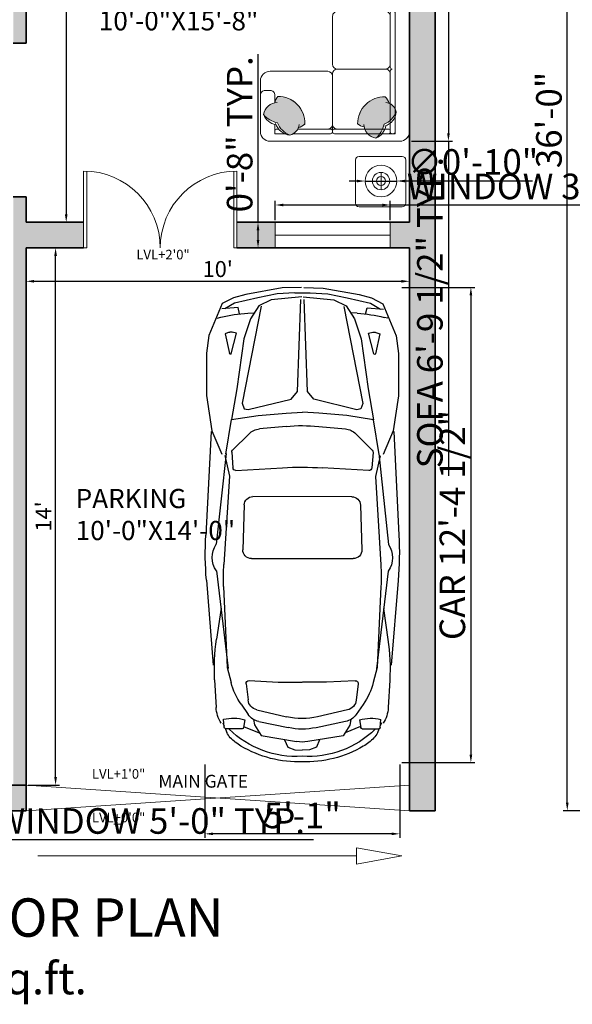
# Model space of a CAD drawing. Units: inches. Extents: x 3259 to 4981, y 1402 to 2026.
# Tile 2 of 11: x 3471 to 3644, y 1415 to 1722. Entities that reach past the tile are written whole.
import ezdxf

# ---------------------------------------------------------------- set-up
doc = ezdxf.new("R2010")
doc.units = ezdxf.units.IN
for name, color, linetype, lineweight in [('A-ANNO-DIMS', 2, 'Continuous', 13), ('A-ANNO-SYMB', 7, 'Continuous', 13), ('A-ANNO-TEXT', 7, 'Continuous', 18), ('A-ANNO-TITL', 7, 'Continuous', 25), ('A-AREA-IDEN', 7, 'Continuous', 18), ('A-DOOR', 3, 'Continuous', 18), ('A-FURN', 8, 'Continuous', 13), ('A-GLAZ', 4, 'Continuous', 18), ('A-VEHI', 8, 'Continuous', 13), ('A-WALL', 7, 'Continuous', 35), ('A-WALL-PATT', 252, 'Continuous', 13)]:
    doc.layers.add(name, color=color, linetype=linetype, lineweight=lineweight)
doc.layers.add('L9012X$0', color=2, linetype='Continuous')
doc.styles.get("Standard").update_dxf_attribs({"font": 'arial.ttf'})
doc.dimstyles.new('ISO-25', dxfattribs={"dimtxt": 8, "dimasz": 2.5, "dimexe": 1.25, "dimexo": 0.625, "dimtad": 1, "dimdec": 1, "dimlunit": 3, "dimtxsty": 'Standard', "dimcen": 2.5, "dimclrd": 4, "dimclre": 4, "dimclrt": 1, "dimadec": 0, "dimazin": 0, "dimtfac": 1, "dimtdec": 1, "dimtmove": 0, "dimatfit": 3, "dimfxl": 1, "dimarcsym": 0})

# ---------------------------------------------------------------- blocks, each defined once
blk = doc.blocks.new('SOFA 1')
at = {"transparency": 33554687}
h = blk.add_hatch(color=256, dxfattribs=at)
h.dxf.hatch_style = 1
h.paths.add_polyline_path([(3723.52, 1308.63, 0.147724), (3717.76, 1305.24, 0.310469), (3722.42, 1300.4), (3722.42, 1300.25, 0.156703), (3723.62, 1297.8, 0.425821), (3734.69, 1309.08, 0.121928), (3732.05, 1310.63, 0.233216), (3728.6, 1313.59, 0.213835)])
h = blk.add_hatch(color=256, dxfattribs=at)
h.dxf.hatch_style = 1
h.paths.add_polyline_path([(3769.65, 1307.6, 0.084911), (3767.15, 1309.12, 0.046133), (3766.46, 1311.13), (3759.18, 1311.13, 0.039409), (3758.92, 1310.24, 0.165523), (3756.31, 1309.02, 0.42585), (3767.59, 1297.95, 0.121928), (3769.15, 1300.58, 0.027403), (3769.65, 1300.83)])
h.paths.add_polyline_path([(3765.34, 1313.08), (3760.4, 1313.08, 0.097704), (3759.18, 1311.13), (3766.46, 1311.13, 0.04873)])
h.paths.add_polyline_path([(3763.76, 1314.88, 0.16488), (3760.4, 1313.08), (3765.34, 1313.08, 0.051917)])
h.paths.add_polyline_path([(3771.6, 1305.17, 0.090388), (3769.65, 1307.6), (3769.65, 1300.83, 0.136035), (3771.6, 1302.77)])
h = blk.add_hatch(color=256, dxfattribs=at)
h.dxf.hatch_style = 1
h.paths.add_polyline_path([(3769.16, 1235.96, 0.122267), (3767.6, 1238.61, 0.425972), (3756.32, 1227.54, 0.165563), (3758.93, 1226.32, 0.309481), (3763.76, 1221.69, 0.002677), (3763.83, 1221.72, 0.146094), (3767.16, 1227.43, 0.212433), (3772.1, 1232.48, 0.235342)])
h = blk.add_hatch(color=256, dxfattribs=at)
h.dxf.hatch_style = 1
h.paths.add_polyline_path([(3769.16, 1225.36, 0.122267), (3767.6, 1228.01, 0.425972), (3756.32, 1216.94, 0.165563), (3758.93, 1215.72, 0.309481), (3763.76, 1211.09, 0.002677), (3763.83, 1211.12, 0.146094), (3767.16, 1216.83, 0.212433), (3772.1, 1221.88, 0.235342)])
for p, q in [((3720.45, 1316.13), (3773.58, 1316.13)), ((3777.51, 1312.19), (3777.51, 1213.72))]:
    blk.add_line(p, q, dxfattribs=at)
for points in [[(3717.76, 1305.24, -0.147724), (3723.52, 1308.63, -0.213355), (3728.59, 1313.59, 0.213355), (3723.52, 1308.63, 0.147724), (3717.76, 1305.24, -0.249545), (3722.86, 1309.34, 0.249545), (3717.75, 1305.25, 0.356779), (3723.4, 1300.28, -0.356779), (3717.76, 1305.24)], [(3728.58, 1313.6, -0.306333), (3732.42, 1309.31, 0.306333), (3728.58, 1313.6, 0.306674), (3722.72, 1308.89, -0.306674), (3728.58, 1313.6)], [(3763.76, 1314.88, -0.147724), (3767.15, 1309.12, -0.213355), (3772.1, 1304.05, 0.213355), (3767.15, 1309.12, 0.147724), (3763.76, 1314.88, -0.249545), (3767.86, 1309.77, 0.249545), (3763.77, 1314.89, 0.356779), (3758.8, 1309.23, -0.356779), (3763.76, 1314.88)], [(3734.69, 1309.08, -0.425972), (3723.62, 1297.8, -0.165552), (3722.4, 1300.4, 0.165552), (3723.62, 1297.79, 0.425972), (3734.69, 1309.07, 0.121514), (3732.07, 1310.63, -0.121514), (3734.69, 1309.08)], [(3767.6, 1297.95, -0.425972), (3756.31, 1309.01, -0.165552), (3758.92, 1310.24, 0.165552), (3756.31, 1309.02, 0.425972), (3767.59, 1297.95, 0.121514), (3769.14, 1300.57, -0.121514), (3767.6, 1297.95)], [(3772.11, 1304.06, -0.306333), (3767.83, 1300.22, 0.306333), (3772.11, 1304.06, 0.306674), (3767.4, 1309.91, -0.306674), (3772.11, 1304.06)], [(3770.44, 1286.63, -0.414214), (3769.66, 1287.4, 0.414214), (3770.44, 1286.63, 0.414214), (3769.66, 1285.83, -0.414214), (3770.44, 1286.63)], [(3748.01, 1262.99, -0.414214), (3746.05, 1264.95, 0.414214), (3748.01, 1262.97, 0.414213), (3746.05, 1261.01, -0.414213), (3748.01, 1262.99)], [(3770.44, 1262.99, -0.414214), (3769.66, 1263.77, 0.414214), (3770.44, 1262.99, 0.414214), (3769.66, 1262.19, -0.414214), (3770.44, 1262.99)], [(3770.83, 1262.97, -0.414214), (3771.61, 1262.19, 0.414214), (3770.83, 1262.99, 0.414214), (3771.61, 1263.77, -0.414214), (3770.83, 1262.97)], [(3748.01, 1239.35, -0.414214), (3746.05, 1241.31, 0.414214), (3748.01, 1239.33, 0.414213), (3746.05, 1237.37, -0.414213), (3748.01, 1239.35)], [(3767.7, 1239.33, -0.414214), (3769.66, 1237.37, 0.414214), (3767.7, 1239.35, 0.414214), (3769.66, 1241.31, -0.414214), (3767.7, 1239.33)], [(3756.32, 1227.54, -0.425972), (3767.6, 1238.61, -0.121514), (3769.16, 1235.98, 0.121514), (3767.6, 1238.61, 0.425972), (3756.32, 1227.54, 0.165552), (3758.93, 1226.32, -0.165552), (3756.32, 1227.54)], [(3770.44, 1239.35, -0.414214), (3769.66, 1240.13, 0.414214), (3770.44, 1239.33, 0.414214), (3769.66, 1238.55, -0.414214), (3770.44, 1239.35)], [(3770.83, 1239.33, -0.414214), (3771.61, 1238.55, 0.414214), (3770.83, 1239.35, 0.414214), (3771.61, 1240.13, -0.414214), (3770.83, 1239.33)], [(3763.78, 1221.67, 0.249545), (3767.87, 1226.78, -0.249545), (3763.76, 1221.69, -0.356779), (3758.81, 1227.32, 0.356779), (3763.77, 1221.68, 0.147724), (3767.16, 1227.43, 0.213355), (3772.11, 1232.51, -0.213355), (3767.16, 1227.43, -0.147724), (3763.78, 1221.67)], [(3772.1, 1232.5, -0.306674), (3767.41, 1226.64, 0.306674), (3772.1, 1232.5, 0.306333), (3767.84, 1236.34, -0.306333), (3772.1, 1232.5)], [(3756.32, 1216.94, -0.200233), (3759.49, 1224.76, 0.200233), (3756.32, 1216.94, 0.165552), (3758.93, 1215.72, -0.165552), (3756.32, 1216.94)], [(3772.1, 1221.9, -0.306674), (3767.41, 1216.04, 0.306674), (3772.1, 1221.9, -0.213355), (3767.16, 1216.83, -0.147724), (3763.77, 1211.08, 0.147724), (3767.15, 1216.83, 0.213355), (3772.1, 1221.9)], [(3763.76, 1211.09, -0.356779), (3758.81, 1216.72, 0.356779), (3763.76, 1211.09, 0.249545), (3767.87, 1216.18, -0.249545), (3763.76, 1211.09)]]:
    blk.add_lwpolyline(points, format="xyb", dxfattribs=at)
for points in [[(3722.42, 1313.08), (3722.42, 1309.23), (3722.42, 1313.08), (3726.57, 1313.08)], [(3729.85, 1313.08), (3745.25, 1313.08)], [(3768.11, 1313.08), (3746.78, 1313.08)], [(3771.6, 1313.08), (3767.75, 1313.08), (3771.6, 1313.08), (3771.6, 1308.93)], [(3771.6, 1313.08), (3771.61, 1233.74)], [(3716.51, 1312.2), (3716.51, 1291.44)], [(3723.21, 1311.13), (3723.93, 1311.13)], [(3731.82, 1311.13), (3745.25, 1311.13)], [(3746.01, 1312.3), (3746.01, 1288.55)], [(3746.01, 1310.97), (3746.01, 1311.36)], [(3768.87, 1311.13), (3746.78, 1311.13)], [(3769.66, 1287.39), (3769.65, 1312.3)], [(3769.65, 1309.43), (3769.65, 1308.71)], [(3746.01, 1288.54), (3746.01, 1308.23)], [(3722.42, 1300.39), (3722.42, 1297.33)], [(3720.45, 1295.38), (3718.48, 1295.38)], [(3720.45, 1287.5), (3744.09, 1287.5)], [(3747.99, 1286.6), (3767.69, 1286.6)], [(3769.66, 1263.75), (3769.66, 1285.81)], [(3746.02, 1284.63), (3746.02, 1264.94)], [(3769.66, 1277.18), (3769.66, 1263.75)], [(3746.02, 1260.99), (3746.02, 1241.3)], [(3747.99, 1262.97), (3767.69, 1262.97)], [(3769.66, 1240.12), (3769.66, 1262.18)], [(3770.43, 1262.97), (3770.82, 1262.97)], [(3746.02, 1237.36), (3746.02, 1213.74)], [(3747.99, 1239.33), (3767.69, 1239.33)], [(3769.66, 1235.71), (3769.66, 1238.54)], [(3770.43, 1239.33), (3770.82, 1239.33)], [(3771.61, 1223.14), (3771.61, 1230.47)], [(3769.66, 1225.11), (3769.66, 1227.82)], [(3767.76, 1215.72), (3771.61, 1215.72), (3771.61, 1219.84), (3771.61, 1215.72)], [(3769.66, 1216.5), (3769.66, 1217.22)], [(3753.91, 1211.77), (3753.91, 1213.74)], [(3755.86, 1215.72), (3758.92, 1215.72)], [(3749.97, 1209.8), (3773.58, 1209.8)]]:
    blk.add_lwpolyline(points, close=True, dxfattribs=at)
for points in [[(3770.43, 1313.08, 0.414214), (3769.65, 1312.3, -0.414214)], [(3771.6, 1312.3, 0.414214), (3770.82, 1313.08, -0.414214)], [(3722.42, 1311.91, 0.414214), (3723.2, 1311.13, -0.414214)], [(3716.51, 1297.34, 0.414214), (3718.47, 1295.38, -0.414214)], [(3720.44, 1295.38, 0.414214), (3722.4, 1297.34, -0.414214)], [(3716.51, 1291.45, 0.414212), (3720.44, 1287.52, -0.414212)], [(3746.03, 1288.56, 0.414214), (3747.99, 1286.6, 0.414213), (3746.03, 1284.64, -0.414213), (3747.99, 1286.6, -0.414214)], [(3769.66, 1284.64, 0.414214), (3767.7, 1286.6, 0.414214), (3769.66, 1288.56, -0.414214), (3767.7, 1286.6, -0.414214)], [(3769.66, 1261.01, 0.414214), (3767.7, 1262.97, 0.414214), (3769.66, 1264.93, -0.414214), (3767.7, 1262.97, -0.414214)], [(3772.13, 1221.9, 0.306333), (3767.84, 1225.74, -0.306333)], [(3769.16, 1225.36, 0.071861), (3768.39, 1227.01, -0.071861)], [(3769.66, 1216.52, 0.414214), (3770.44, 1215.74, -0.414214)], [(3770.83, 1215.74, 0.414214), (3771.61, 1216.52, -0.414214)], [(3746.05, 1213.76, 0.414212), (3749.98, 1209.82, -0.414212)], [(3755.87, 1215.72, 0.414214), (3753.91, 1213.76, -0.414214)], [(3755.87, 1209.8, -0.414214), (3753.91, 1211.76, 0.414214)]]:
    blk.add_lwpolyline(points, format="xyb", close=True, dxfattribs=at)
for centre, radius, start, end in [((3720.44, 1312.2), 3.93, 90.0002, 179.9998), ((3720.44, 1312.19), 3.94, 89.9158, 179.9154), ((3745.22, 1312.29), 0.789, 0.8425, 90.8425), ((3746.8, 1312.29), 0.789, 89.1575, 179.1575), ((3768.87, 1312.3), 0.777, 360, 90), ((3773.58, 1312.2), 3.93, 0.0002, 89.9998), ((3773.57, 1312.19), 3.94, 359.9158, 89.9154), ((3744.09, 1309.21), 1.92, 358.766, 90.5111), ((3745.24, 1311.91), 0.777, 270, 0), ((3745.24, 1311.91), 0.777, 270, 0), ((3746.79, 1311.91), 0.777, 180, 270), ((3746.79, 1311.91), 0.777, 180, 270), ((3747.93, 1309.21), 1.92, 89.4889, 181.234), ((3768.87, 1311.91), 0.777, 270, 0), ((3744.08, 1289.48), 1.96, 270, 360), ((3744.08, 1289.48), 1.96, 270, 360), ((3773.58, 1213.73), 3.93, 270.0002, 359.9998), ((3773.59, 1213.73), 3.93, 269.9156, 359.9152)]:
    blk.add_arc(centre, radius, start, end, dxfattribs=at)
blk = doc.blocks.new('A1099DC')
at = {"color": 0, "linetype": 'ByBlock'}
for p, q in [((1279.298465, 804.448389), (2201.430588, 851.890505)), ((2602.736326, 846.078152), (3356.693814, 785.353187)), ((179.200345, 564.515703), (190.951238, 709.631982)), ((272.228253, 749.073842), (265.114727, 718.465169)), ((1475.52921, 670.226262), (2282.402739, 758.004075)), ((2519.280414, 756.817792), (3387.476361, 653.818028)), ((2851.341839, 715.213377), (3126.60716, 755.701993)), ((3488.458929, 772.663345), (3732.658862, 759.86454)), ((3867.794139, 700.329656), (3900.059395, 686.767505)), ((139.051458, 595.027331), (190.951238, 683.213377)), ((405.405047, 577.538958), (396.874865, 615.894428)), ((398.733388, 644.315148), (411.280494, 678.748261)), ((589.014326, 626.599587), (405.405047, 577.538958)), ((411.280494, 678.748261), (588.616917, 641.417897)), ((1482.852352, 674.283145), (1175.286956, 622.180789)), ((1300.814287, 466.658131), (1445.712032, 613.104998)), ((1465.665584, 620.56924), (1602.893878, 610.287296)), ((1494.603245, 682.841284), (1678.210958, 641.166865)), ((1678.210958, 641.166865), (2462.684993, 690.847736)), ((2656.476214, 692.831247), (3376.704709, 662.004075)), ((3376.704709, 662.004075), (3510.708679, 626.736433)), ((3909.27561, 688.812956), (3837.725727, 693.401722)), ((3921.162781, 527.618662), (3921.162781, 676.138994)), ((3925.383812, 676.122818), (3955.306409, 663.545364)), ((92.537504, 388.14361), (139.051458, 595.027331)), ((236.043912, 551.980927), (179.200345, 564.515703)), ((1626.354615, 583.507504), (1602.652901, 169.222264)), ((3704.596898, 536.993674), (3795.675135, 473.385795)), ((229.117398, 477.634662), (225.714299, 427.957563)), ((1933.148906, 509.557888), (2330.980062, 522.200075)), ((2409.60024, 445.938054), (2410.49349, -460.09121)), ((3493.960271, 465.734554), (3507.923021, 209.166865)), ((3522.252709, 492.345257), (3666.066199, 475.644444)), ((3841.786866, 503.451367), (3910.58243, 515.096797)), ((3901.001848, 514.780764), (3957.150905, 375.772812)), ((57.774444, 216.608726), (92.537504, 388.14361)), ((1235.045743, 136.116317), (1257.419842, 373.755108)), ((1860.238743, -448.635916), (1859.369151, 433.397797)), ((3753.293176, 397.789551), (3815.226005, 132.124765)), ((3839.396146, 426.841284), (3888.358202, 417.538958)), ((3857.610793, 379.525702), (3912.067615, 118.157673)), ((3888.358202, 417.538958), (3983.199613, 359.957848)), ((3983.199613, 359.957848), (4035.448301, 43.94997)), ((49.168662, 58.00681), (57.774444, 216.608726)), ((3507.923021, 209.166865), (3507.64153, -4.333678)), ((4019.086894, 150.376168), (4084.69605, 122.469191)), ((4084.69605, 122.469191), (4109.177079, 60.329656)), ((4109.177079, 60.329656), (4113.094043, -5.158716)), ((49.301278, -76.507426), (58.219773, -235.092064)), ((3508.347273, -221.154823), (3507.644805, -7.65525)), ((3983.920268, -371.008369), (4035.545755, -54.898082)), ((4084.948231, -133.320044), (4109.306686, -71.132359)), ((4109.306686, -71.132359), (4113.094514, -5.636391)), ((1235.330373, -152.586046), (1258.173002, -390.180259)), ((3754.088875, -409.293325), (3815.497749, -143.506937)), ((3858.370276, -390.823819), (3912.311631, -129.348921)), ((4019.394229, -161.356334), (4084.948231, -133.320044)), ((58.219773, -235.092064), (93.320996, -406.558069)), ((1627.520644, -599.204785), (1603.002095, -184.967086)), ((3494.890446, -477.749545), (3508.347273, -221.154823)), ((93.320996, -406.558069), (140.24279, -613.349673)), ((3840.248961, -438.175225), (3889.19258, -428.776374)), ((3889.19258, -428.776374), (3983.920268, -371.008369)), ((3902.027941, -525.993061), (3957.902795, -386.874665)), ((230.077082, -495.779641), (226.576036, -446.109349)), ((1301.750547, -482.997536), (1446.936772, -629.158411)), ((1934.168526, -524.650381), (2332.023837, -536.508105)), ((3523.2353, -504.304409), (3667.01558, -487.320059)), ((3705.667171, -548.593196), (3796.61981, -484.805853)), ((3842.790735, -514.780444), (3911.609128, -526.290202)), ((237.150178, -570.112104), (180.331436, -582.758939)), ((180.331436, -582.758939), (192.368445, -727.851766)), ((406.561378, -595.336142), (398.106841, -633.708356)), ((590.267037, -644.034637), (406.561378, -595.336142)), ((3922.214148, -538.79118), (3922.506998, -687.311224)), ((140.24279, -613.349673), (192.316354, -701.433212)), ((400.0214, -662.125356), (412.636377, -696.533662)), ((412.636377, -696.533662), (589.898847, -658.853701)), ((1484.19765, -690.263206), (1176.530118, -638.767405)), ((1466.905004, -636.583294), (1604.112757, -626.030785)), ((1476.866524, -686.22077), (2283.911563, -772.40743)), ((1495.965396, -698.798158), (1679.490579, -656.761786)), ((1679.490579, -656.761786), (2464.061049, -704.895745)), ((2520.786439, -770.754078), (3388.777604, -666.042617)), ((2657.855804, -706.497136), (3378.022114, -674.249887)), ((3378.022114, -674.249887), (3511.956283, -638.718087)), ((3869.186159, -711.60707), (3901.424611, -697.981326)), ((3926.727989, -687.286725), (3956.625729, -674.650294)), ((273.723073, -767.133288), (266.549207, -736.538701)), ((2852.765183, -728.494989), (3128.109803, -768.440762)), ((3489.994314, -784.688586), (3734.168535, -771.408296)), ((3910.644841, -700.0086), (3839.104145, -704.738438)), ((1280.900818, -820.829563), (2203.124693, -866.453338)), ((2604.418191, -859.849707), (3358.254477, -797.638217))]:
    blk.add_line(p, q, dxfattribs=at)
for points in [[(-0.000783, 0.794772), (5.385043, 172.701749), (63.649891, 493.818028), (92.537504, 603.957563), (144.437284, 705.166865), (428.417214, 824.236633), (585.095796, 846.190121), (961.406447, 846.190121), (1274.27399, 797.818028), (1482.852352, 709.631982)], [(83.345007, -3.206171), (111.32237, 268.957533), (164.563706, 379.583828), (279.999271, 453.709838), (456.549665, 511.628518), (901.254996, 574.918954), (1175.286956, 622.180789), (1137.52997, 385.548359), (1118.345181, 137.317882), (1109.829198, -8.358455)], [(168.178729, 359.003083), (1030.214866, 528.397865), (1077.798844, 510.531569), (1086.170082, 475.285426), (992.832238, 91.960378), (924.218938, 35.478085), (108.447994, 6.034416)], [(0.019119, -19.392451), (5.743899, -191.288474), (64.641806, -512.289243), (93.746535, -622.371603), (145.845778, -723.478374), (430.059935, -841.987962), (586.7815, -863.632471), (963.091723, -863.198028), (1275.863278, -814.209121), (1484.26735, -725.611974)], [(83.356858, -15.227176), (111.870816, -287.335185), (165.330179, -397.856284), (280.911681, -471.754535), (457.575935, -529.324983), (902.4055, -592.045995), (1176.530118, -638.767405), (1138.306616, -402.209884), (1118.632407, -154.017717), (1109.829198, -8.358455)], [(168.904615, -377.268451), (1031.273389, -545.270714), (1078.822046, -527.310627), (1087.123771, -492.048047), (993.030273, -108.907787), (924.305735, -52.560894), (108.478017, -24.418246)]]:
    blk.add_lwpolyline(points, dxfattribs=at)
for centre, radius, start, end in [((2358.037832, -2192.08357), 3048, 85.395244, 92.945173), ((2399.99649, 588.663508), 206.166238, 54.649181, 124.776949), ((1749.553982, 373.478072), 1524, 166.916578, 176.08111), ((3392.740754, -1053.630025), 1828.8, 86.999806, 98.367602), ((3718.678317, 475.802507), 284.405862, 57.329946, 87.182375), ((446.46332, 626.922805), 50.8, 159.97873, 192.538409), ((587.047263, 633.961317), 7.62, 284.960009, 78.112462), ((1463.767788, 595.240237), 25.4, 85.715073, 135.304647), ((2578.271641, -1134.295865), 1828.8, 87.549126, 93.623712), ((3355.555414, 37.211519), 609.6, 55.070043, 75.255062), ((4191.049821, 605.937201), 363.988953, 166.096081, 196.353514), ((3908.462781, 676.138994), 12.7, 0, 86.330429), ((3320.85101, 50.338397), 847.430844, 356.245089, 44.519453), ((3896.252417, 523.051998), 152.4, 46.38363, 67.20138), ((3700.933354, 318.064082), 435.542335, 30.457681, 46.38363), ((1600.996082, 584.958293), 25.4, 356.725615, 85.715073), ((3908.462781, 527.618662), 12.7, 279.607718, 0), ((3204.184594, 25.950693), 1011.814461, 358.069446, 30.457681), ((1409.148822, 359.469565), 152.4, 135.304647, 174.62136), ((1935.569151, 433.396333), 76.2, 91.82012, 179.9989), ((2333.400307, 446.03852), 76.2, 359.924458, 91.82012), ((3519.322741, 467.114813), 25.4, 83.37601, 183.115039), ((3654.346327, 374.722669), 101.6, 13.122645, 83.37601), ((3708.414764, 348.440256), 152.4, 11.769371, 55.070043), ((2752.335538, -6.739118), 1524, 174.62136, 185.491615), ((4645.676894, -4.872483), 3048, 176.725615, 183.38736), ((3221.54491, -6.276527), 609.6, 346.99033, 13.122645), ((3315.283499, -6.18411), 609.6, 348.343604, 11.769371), ((1266.577845, -8.050136), 1219.2, 176.894161, 183.218814), ((3734.73098, -5.770579), 304.8, 350.724636, 9.388339), ((3320.962449, -62.69553), 847.430844, 315.593523, 3.867886), ((3204.248172, -38.537915), 1011.814461, 329.655294, 2.043529), ((1409.873518, -375.595566), 152.4, 185.491615, 224.808328), ((3655.096735, -386.42159), 101.6, 276.736965, 346.99033), ((3709.113243, -360.032616), 152.4, 305.042932, 348.343604), ((1750.305335, -388.625277), 1524, 184.031865, 193.196397), ((1936.438592, -448.484202), 76.2, 180.114076, 268.292856), ((2334.293902, -460.341926), 76.2, 268.292856, 0.188517), ((3520.255588, -479.079792), 25.4, 176.997936, 276.736965), ((4192.255091, -616.577407), 363.988953, 163.759461, 194.016894), ((1602.165021, -600.705574), 25.4, 274.397903, 3.38736), ((3355.640902, -49.500248), 609.6, 284.857913, 305.042932), ((3909.514173, -538.816222), 12.7, 0.112975, 80.505257), ((3701.571953, -329.671253), 435.542335, 313.729345, 329.655294), ((447.716945, -644.638934), 50.8, 167.574566, 200.134245), ((588.314493, -651.400231), 7.62, 282.000513, 75.152966), ((1464.957267, -611.258083), 25.4, 224.808328, 274.397903), ((3909.807023, -687.336265), 12.7, 273.782546, 0.112975), ((3897.294828, -534.273643), 152.4, 292.911596, 313.729345), ((2401.171182, -602.835323), 206.166238, 235.336026, 305.463794), ((2576.048678, 1120.472221), 1828.8, 266.489263, 272.563849), ((3390.675263, 1041.412497), 1828.8, 261.745373, 273.113169), ((3719.627907, -487.374382), 284.405862, 272.930601, 302.78303), ((2353.729565, 2177.823616), 3048, 267.167802, 274.717731)]:
    blk.add_arc(centre, radius, start, end, dxfattribs=at)
blk = doc.blocks.new('VI')
at = {"layer": 'L9012X$0'}
blk.add_blockref('A1099DC', (0, 0), dxfattribs=at)
blk = doc.blocks.new('table-31')
at = {"color": 0, "linetype": 'ByBlock'}
for p, q in [((-0.2031, 0.1666), (-0.2031, -0.1763)), ((0.1683, 0.1952), (-0.1746, 0.1952)), ((0.1969, 0.1666), (0.1969, -0.1763)), ((-0.0689, 0), (0.0689, 0)), ((0, -0.0689), (0, 0.0689)), ((0.1683, -0.2048), (-0.1746, -0.2048))]:
    blk.add_line(p, q, dxfattribs=at)
for radius in [0.1261, 0.0689, 0.0353]:
    blk.add_circle((0, 0), radius, dxfattribs=at)
for centre, start, end in [((-0.1746, 0.1666), 90, 180), ((0.1683, 0.1666), 0, 90), ((-0.1746, -0.1763), 180, 270), ((0.1683, -0.1763), 270, 0)]:
    blk.add_arc(centre, 0.0286, start, end, dxfattribs=at)
blk = doc.blocks.new('*D26')
at = {"layer": 'A-ANNO-DIMS', "color": 0, "lineweight": -2, "transparency": 16777216}
for p, q in [((3473.79, 1847.12), (3486.99, 1847.12)), ((3485.74, 1844.62), (3485.74, 1661.62)), ((3473.79, 1659.12), (3486.99, 1659.12))]:
    blk.add_line(p, q, dxfattribs=at)
at = {"layer": 'A-ANNO-DIMS', "color": 0, "transparency": 16777216}
for points in [[(3485.32, 1844.62), (3486.16, 1844.62), (3485.74, 1847.12)], [(3485.32, 1661.62), (3486.16, 1661.62), (3485.74, 1659.12)]]:
    blk.add_solid(points, dxfattribs=at)
at = {"layer": 'Defpoints', "color": 0, "transparency": 16777216}
for p in [(3473.16, 1847.12), (3473.16, 1659.12), (3485.74, 1659.12)]:
    blk.add_point(p, dxfattribs=at)
at = {"layer": 'A-ANNO-DIMS', "color": 0, "transparency": 16777216, "insert": (3482.56, 1753.12), "char_height": 5, "attachment_point": 5, "rotation": 90}
blk.add_mtext('15\'-8"', dxfattribs=at)
blk = doc.blocks.new('*D33')
at = {"layer": 'A-ANNO-DIMS', "color": 0, "lineweight": -2, "transparency": 16777216}
for p, q in [((3473.79, 1651.12), (3483.66, 1651.12)), ((3482.41, 1485.62), (3482.41, 1648.62)), ((3473.79, 1483.12), (3483.66, 1483.12))]:
    blk.add_line(p, q, dxfattribs=at)
at = {"layer": 'A-ANNO-DIMS', "color": 0, "transparency": 16777216}
for points in [[(3481.99, 1648.62), (3482.82, 1648.62), (3482.41, 1651.12)], [(3481.99, 1485.62), (3482.82, 1485.62), (3482.41, 1483.12)]]:
    blk.add_solid(points, dxfattribs=at)
at = {"layer": 'Defpoints', "color": 0, "transparency": 16777216}
for p in [(3473.16, 1651.12), (3482.41, 1651.12), (3473.16, 1483.12)]:
    blk.add_point(p, dxfattribs=at)
at = {"layer": 'A-ANNO-DIMS', "color": 0, "transparency": 16777216, "insert": (3479.27, 1567.12), "char_height": 5, "attachment_point": 5, "rotation": 90}
blk.add_mtext("14'", dxfattribs=at)
blk = doc.blocks.new('*D34')
at = {"layer": 'A-ANNO-DIMS', "color": 0, "lineweight": -2, "transparency": 16777216}
for p, q in [((3473.16, 1650.49), (3473.16, 1639.41)), ((3593.16, 1650.49), (3593.16, 1639.41)), ((3475.66, 1640.66), (3590.66, 1640.66))]:
    blk.add_line(p, q, dxfattribs=at)
at = {"layer": 'A-ANNO-DIMS', "color": 0, "transparency": 16777216}
for points in [[(3475.66, 1641.08), (3475.66, 1640.25), (3473.16, 1640.66)], [(3590.66, 1641.08), (3590.66, 1640.25), (3593.16, 1640.66)]]:
    blk.add_solid(points, dxfattribs=at)
at = {"layer": 'Defpoints', "color": 0, "transparency": 16777216}
for p in [(3473.16, 1651.12), (3593.16, 1651.12), (3593.16, 1640.66)]:
    blk.add_point(p, dxfattribs=at)
at = {"layer": 'A-ANNO-DIMS', "color": 0, "transparency": 16777216, "insert": (3533.16, 1643.84), "char_height": 5, "attachment_point": 5}
blk.add_mtext("10'", dxfattribs=at)
blk = doc.blocks.new('ENTRY-DOOR-PAIR-48IN')
for p, q in [((0, 0), (0, 24)), ((1, 0), (1, 24)), ((47, 0), (47, 24)), ((48, 0), (48, 24)), ((0, 0), (0, 8)), ((48, 0), (48, 8)), ((0, 0), (1, 0)), ((48, 0), (47, 0))]:
    blk.add_line(p, q)
for centre, start, end in [((0, 0), 0, 90), ((48, 0), 90, 180)]:
    blk.add_arc(centre, 24, start, end)
blk = doc.blocks.new('PARKING-GATE-120IN')
for p, q in [((0, 8), (120, 0)), ((120, 8), (0, 0))]:
    blk.add_line(p, q)
blk = doc.blocks.new('WINDOW-36x8')
for p, q in [((0, 0), (0, 8)), ((36, 0), (36, 8)), ((0, 4), (36, 4))]:
    blk.add_line(p, q)
blk = doc.blocks.new('ROAD-DIRECTION')
blk.add_line((99.82, 2.55), (0, 2.55))
blk.add_lwpolyline([(113.98, 2.55), (99.82, 5.11), (99.82, 0)], close=True)
blk = doc.blocks.new('*D156')
at = {"layer": 'A-ANNO-DIMS', "color": 4, "lineweight": -2, "transparency": 16777216}
for p, q in [((3593.79, 1765.74), (3606.61, 1765.74)), ((3605.36, 1763.24), (3605.36, 1686.95)), ((3593.79, 1684.45), (3606.61, 1684.45)), ((3605.36, 1684.45), (3605.36, 1579.8))]:
    blk.add_line(p, q, dxfattribs=at)
at = {"layer": 'A-ANNO-DIMS', "color": 4, "transparency": 16777216}
for points in [[(3604.94, 1763.24), (3605.78, 1763.24), (3605.36, 1765.74)], [(3604.94, 1686.95), (3605.78, 1686.95), (3605.36, 1684.45)]]:
    blk.add_solid(points, dxfattribs=at)
at = {"layer": 'Defpoints', "color": 0, "transparency": 16777216}
for p in [(3593.17, 1765.74), (3593.17, 1684.45), (3605.36, 1684.45)]:
    blk.add_point(p, dxfattribs=at)
at = {"layer": 'A-ANNO-DIMS', "color": 1, "transparency": 16777216, "insert": (3600.6, 1630.88), "char_height": 8, "attachment_point": 5, "rotation": 90}
blk.add_mtext('SOFA 6\'-9 1/2" TYP.', dxfattribs=at)
blk = doc.blocks.new('*D174')
at = {"layer": 'A-ANNO-DIMS', "color": 4, "lineweight": -2, "transparency": 16777216}
for p, q in [((3398.16, 1474.49), (3398.16, 1464.87)), ((3458.16, 1474.49), (3458.16, 1464.87)), ((3400.66, 1466.12), (3455.66, 1466.12)), ((3458.16, 1466.12), (3563.15, 1466.12))]:
    blk.add_line(p, q, dxfattribs=at)
at = {"layer": 'A-ANNO-DIMS', "color": 4, "transparency": 16777216}
for points in [[(3400.66, 1466.53), (3400.66, 1465.7), (3398.16, 1466.12)], [(3455.66, 1466.53), (3455.66, 1465.7), (3458.16, 1466.12)]]:
    blk.add_solid(points, dxfattribs=at)
at = {"layer": 'Defpoints', "color": 0, "transparency": 16777216}
for p in [(3398.16, 1475.12), (3458.16, 1475.12), (3458.16, 1466.12)]:
    blk.add_point(p, dxfattribs=at)
at = {"layer": 'A-ANNO-DIMS', "color": 1, "transparency": 16777216, "insert": (3511.91, 1470.88), "char_height": 8, "attachment_point": 5}
blk.add_mtext('WINDOW 5\'-0" TYP.', dxfattribs=at)
blk = doc.blocks.new('*D175')
at = {"layer": 'A-ANNO-DIMS', "color": 4, "lineweight": -2, "transparency": 16777216}
for p, q in [((3467.16, 1483.12), (3467.16, 1535.63)), ((3458.79, 1483.12), (3468.41, 1483.12)), ((3467.16, 1477.62), (3467.16, 1480.62)), ((3458.79, 1475.12), (3468.41, 1475.12))]:
    blk.add_line(p, q, dxfattribs=at)
at = {"layer": 'A-ANNO-DIMS', "color": 4, "transparency": 16777216}
for points in [[(3466.75, 1480.62), (3467.58, 1480.62), (3467.16, 1483.12)], [(3466.75, 1477.62), (3467.58, 1477.62), (3467.16, 1475.12)]]:
    blk.add_solid(points, dxfattribs=at)
at = {"layer": 'Defpoints', "color": 0, "transparency": 16777216}
for p in [(3458.16, 1483.12), (3467.16, 1483.12), (3458.16, 1475.12)]:
    blk.add_point(p, dxfattribs=at)
at = {"layer": 'A-ANNO-DIMS', "color": 1, "transparency": 16777216, "insert": (3462.45, 1510.62), "char_height": 8, "attachment_point": 5, "rotation": 90}
blk.add_mtext('0\'-8" TYP.', dxfattribs=at)
blk = doc.blocks.new('*D176')
at = {"layer": 'A-ANNO-DIMS', "color": 4, "lineweight": -2, "transparency": 16777216}
for p, q in [((3551.16, 1659.74), (3551.16, 1665.77)), ((3587.16, 1659.74), (3587.16, 1665.77)), ((3553.66, 1664.52), (3584.66, 1664.52)), ((3587.16, 1664.52), (3692.15, 1664.52))]:
    blk.add_line(p, q, dxfattribs=at)
at = {"layer": 'A-ANNO-DIMS', "color": 4, "transparency": 16777216}
for points in [[(3553.66, 1664.93), (3553.66, 1664.1), (3551.16, 1664.52)], [(3584.66, 1664.93), (3584.66, 1664.1), (3587.16, 1664.52)]]:
    blk.add_solid(points, dxfattribs=at)
at = {"layer": 'Defpoints', "color": 0, "transparency": 16777216}
for p in [(3587.16, 1664.52), (3551.16, 1659.12), (3587.16, 1659.12)]:
    blk.add_point(p, dxfattribs=at)
at = {"layer": 'A-ANNO-DIMS', "color": 1, "transparency": 16777216, "insert": (3640.91, 1669.28), "char_height": 8, "attachment_point": 5}
blk.add_mtext('WINDOW 3\'-0" TYP.', dxfattribs=at)
blk = doc.blocks.new('*D177')
at = {"layer": 'A-ANNO-DIMS', "color": 4, "lineweight": -2, "transparency": 16777216}
for p, q in [((3545.76, 1659.12), (3545.76, 1711.63)), ((3550.54, 1659.12), (3544.51, 1659.12)), ((3545.76, 1653.62), (3545.76, 1656.62)), ((3550.54, 1651.12), (3544.51, 1651.12))]:
    blk.add_line(p, q, dxfattribs=at)
at = {"layer": 'A-ANNO-DIMS', "color": 4, "transparency": 16777216}
for points in [[(3545.35, 1656.62), (3546.18, 1656.62), (3545.76, 1659.12)], [(3545.35, 1653.62), (3546.18, 1653.62), (3545.76, 1651.12)]]:
    blk.add_solid(points, dxfattribs=at)
at = {"layer": 'Defpoints', "color": 0, "transparency": 16777216}
for p in [(3545.76, 1659.12), (3551.16, 1659.12), (3551.16, 1651.12)]:
    blk.add_point(p, dxfattribs=at)
at = {"layer": 'A-ANNO-DIMS', "color": 1, "transparency": 16777216, "insert": (3541.05, 1686.62), "char_height": 8, "attachment_point": 5, "rotation": 90}
blk.add_mtext('0\'-8" TYP.', dxfattribs=at)
blk = doc.blocks.new('*D178')
at = {"layer": 'A-ANNO-DIMS', "color": 4, "lineweight": -2, "transparency": 16777216}
for p, q in [((3590.73, 1638.76), (3613.64, 1638.76)), ((3612.39, 1636.26), (3612.39, 1492.68)), ((3590.73, 1490.18), (3613.64, 1490.18))]:
    blk.add_line(p, q, dxfattribs=at)
at = {"layer": 'A-ANNO-DIMS', "color": 4, "transparency": 16777216}
for points in [[(3611.97, 1636.26), (3612.81, 1636.26), (3612.39, 1638.76)], [(3611.97, 1492.68), (3612.81, 1492.68), (3612.39, 1490.18)]]:
    blk.add_solid(points, dxfattribs=at)
at = {"layer": 'Defpoints', "color": 0, "transparency": 16777216}
for p in [(3590.1, 1638.76), (3590.1, 1490.18), (3612.39, 1490.18)]:
    blk.add_point(p, dxfattribs=at)
at = {"layer": 'A-ANNO-DIMS', "color": 1, "transparency": 16777216, "insert": (3607.63, 1564.47), "char_height": 8, "attachment_point": 5, "rotation": 90}
blk.add_mtext('CAR 12\'-4 1/2"', dxfattribs=at)
blk = doc.blocks.new('*D179')
at = {"layer": 'A-ANNO-DIMS', "color": 4, "lineweight": -2, "transparency": 16777216}
for p, q in [((3529.16, 1489.56), (3529.16, 1466.65)), ((3590.1, 1489.56), (3590.1, 1466.65)), ((3587.6, 1467.9), (3531.66, 1467.9))]:
    blk.add_line(p, q, dxfattribs=at)
at = {"layer": 'A-ANNO-DIMS', "color": 4, "transparency": 16777216}
for points in [[(3531.66, 1468.31), (3531.66, 1467.48), (3529.16, 1467.9)], [(3587.6, 1468.31), (3587.6, 1467.48), (3590.1, 1467.9)]]:
    blk.add_solid(points, dxfattribs=at)
at = {"layer": 'Defpoints', "color": 0, "transparency": 16777216}
for p in [(3529.16, 1490.18), (3590.1, 1490.18), (3529.16, 1467.9)]:
    blk.add_point(p, dxfattribs=at)
at = {"layer": 'A-ANNO-DIMS', "color": 1, "transparency": 16777216, "insert": (3559.63, 1472.61), "char_height": 8, "attachment_point": 5}
blk.add_mtext('5\'-1"', dxfattribs=at)
blk = doc.blocks.new('*D187')
at = {"layer": 'A-ANNO-DIMS', "color": 4, "lineweight": -2, "transparency": 16777216}
for p, q in [((3667.04, 1907.12), (3641.31, 1907.12)), ((3642.56, 1477.62), (3642.56, 1904.62)), ((3667.04, 1475.12), (3641.31, 1475.12))]:
    blk.add_line(p, q, dxfattribs=at)
at = {"layer": 'A-ANNO-DIMS', "color": 4, "transparency": 16777216}
for points in [[(3642.15, 1904.62), (3642.98, 1904.62), (3642.56, 1907.12)], [(3642.15, 1477.62), (3642.98, 1477.62), (3642.56, 1475.12)]]:
    blk.add_solid(points, dxfattribs=at)
at = {"layer": 'Defpoints', "color": 0, "transparency": 16777216}
for p in [(3642.56, 1907.12), (3667.66, 1907.12), (3667.66, 1475.12)]:
    blk.add_point(p, dxfattribs=at)
at = {"layer": 'A-ANNO-DIMS', "color": 1, "transparency": 16777216, "insert": (3637.85, 1691.12), "char_height": 8, "attachment_point": 5, "rotation": 90}
blk.add_mtext('36\'-0"', dxfattribs=at)
blk = doc.blocks.new('*D200')
at = {"layer": 'A-ANNO-DIMS', "color": 4, "lineweight": -2, "transparency": 16777216}
for p, q in [((3576.79, 1672.01), (3574.29, 1672.01)), ((3579.29, 1672.01), (3589.22, 1672.01)), ((3631.66, 1672.01), (3591.72, 1672.01))]:
    blk.add_line(p, q, dxfattribs=at)
at = {"layer": 'A-ANNO-DIMS', "color": 4, "transparency": 16777216}
for points in [[(3576.79, 1672.42), (3576.79, 1671.59), (3579.29, 1672.01)], [(3591.72, 1672.42), (3591.72, 1671.59), (3589.22, 1672.01)]]:
    blk.add_solid(points, dxfattribs=at)
at = {"layer": 'Defpoints', "color": 0, "transparency": 16777216}
for p in [(3579.29, 1672.01), (3589.22, 1672.01)]:
    blk.add_point(p, dxfattribs=at)
at = {"layer": 'A-ANNO-DIMS', "color": 1, "transparency": 16777216, "insert": (3612.94, 1676.94), "char_height": 8, "attachment_point": 5, "rotation": 0.0034}
blk.add_mtext('∅0\'-10"', dxfattribs=at)

msp = doc.modelspace()

# ---------------------------------------------------------------- hatches: boundary and pattern name
at = {"layer": 'A-WALL-PATT'}
h = msp.add_hatch(color=256, dxfattribs=at)
h.dxf.hatch_style = 1
h.paths.add_polyline_path([(3601.16, 1907.12), (3301.16, 1907.12), (3301.16, 1475.12), (3398.16, 1475.12), (3398.16, 1483.12), (3309.16, 1483.12), (3309.16, 1579.12), (3421.16, 1579.12), (3421.16, 1583.12), (3309.16, 1583.12), (3309.16, 1721.12), (3433.16, 1721.12), (3433.16, 1725.12), (3309.16, 1725.12), (3309.16, 1899.12), (3345.16, 1899.12), (3345.16, 1881.12), (3349.16, 1881.12), (3349.16, 1899.12), (3429.16, 1899.12), (3429.16, 1887.12), (3433.16, 1887.12), (3433.16, 1899.12), (3505.16, 1899.12), (3505.16, 1887.12), (3509.16, 1887.12), (3509.16, 1899.12), (3593.16, 1899.12), (3593.16, 1851.12), (3539.16, 1851.12), (3539.16, 1847.12), (3593.16, 1847.12), (3593.16, 1659.12), (3587.16, 1659.12), (3587.16, 1651.12), (3593.16, 1651.12), (3593.16, 1475.12), (3601.16, 1475.12)])
h.paths.add_polyline_path([(3433.16, 1863.12), (3429.16, 1863.12), (3429.16, 1851.12), (3345.16, 1851.12), (3345.16, 1847.12), (3382.99, 1847.12), (3382.99, 1847.13), (3383.04, 1847.13), (3383.04, 1847.12), (3387.07, 1847.12), (3387.07, 1847.12), (3387.11, 1847.12), (3433.16, 1847.12)], flags=17)
h.paths.add_polyline_path([(3509.16, 1863.12), (3505.16, 1863.12), (3505.16, 1847.12), (3509.16, 1847.12)], flags=17)
h.paths.add_polyline_path([(3473.16, 1851.12), (3469.16, 1851.12), (3469.16, 1715.12), (3473.16, 1715.12), (3473.16, 1777.43), (3473.16, 1777.43), (3473.16, 1777.47), (3473.16, 1777.47), (3473.16, 1781.5), (3473.16, 1781.5), (3473.16, 1781.55)], flags=17)
h.paths.add_polyline_path([(3491.16, 1659.12), (3473.16, 1659.12), (3473.16, 1667.12), (3469.16, 1667.12), (3469.16, 1483.12), (3473.16, 1483.12), (3473.16, 1651.12), (3491.16, 1651.12)], flags=17)
h.paths.add_polyline_path([(3551.16, 1659.12), (3539.16, 1659.12), (3539.16, 1651.12), (3551.16, 1651.12)], flags=17)
h.paths.add_polyline_path([(3473.16, 1483.12), (3458.16, 1483.12), (3458.16, 1475.12), (3473.16, 1475.12)], flags=17)

# ---------------------------------------------------------------- linework, layer by layer
at = {"layer": 'A-WALL'}
for p, q in [((3473.16, 1715.12), (3473.16, 1851.12)), ((3593.16, 1847.12), (3593.16, 1659.12)), ((3469.16, 1715.12), (3473.16, 1715.12)), ((3469.16, 1667.12), (3473.16, 1667.12)), ((3473.16, 1659.12), (3473.16, 1667.12)), ((3473.16, 1659.12), (3491.16, 1659.12)), ((3539.16, 1659.12), (3593.16, 1659.12)), ((3473.16, 1475.12), (3473.16, 1651.12)), ((3473.16, 1651.12), (3491.16, 1651.12)), ((3539.16, 1651.12), (3593.16, 1651.12)), ((3593.16, 1651.12), (3593.16, 1475.12)), ((3473.16, 1483.12), (3309.16, 1483.12))]:
    msp.add_line(p, q, dxfattribs=at)
msp.add_lwpolyline([(3473.16, 1475.12), (3301.16, 1475.12), (3301.16, 1907.12), (3601.16, 1907.12), (3601.16, 1475.12), (3593.16, 1475.12)], dxfattribs=at)

# ---------------------------------------------------------------- block references
at = {"layer": 'A-ANNO-SYMB'}
msp.add_blockref('ROAD-DIRECTION', (3476.82, 1458.42), dxfattribs=at)
at = {"layer": 'A-DOOR'}
for name, p in [('ENTRY-DOOR-PAIR-48IN', (3491.16, 1651.12)), ('PARKING-GATE-120IN', (3473.16, 1475.12))]:
    msp.add_blockref(name, p, dxfattribs=at)
at = {"layer": 'A-FURN', "xscale": -0.7644053585719659, "yscale": 0.7644053585719659, "zscale": 0.7644053585719659, "rotation": 180}
msp.add_blockref('SOFA 1', (705.61, 2690.51), dxfattribs=at)
at = {"layer": 'A-FURN', "xscale": 39.3701, "yscale": 39.3701, "zscale": 39.3701}
msp.add_blockref('table-31', (3584.26, 1672.01), dxfattribs=at)
at = {"layer": 'A-GLAZ'}
msp.add_blockref('WINDOW-36x8', (3551.16, 1651.12), dxfattribs=at)
at = {"layer": 'A-VEHI', "xscale": -0.0351896714874634, "yscale": 0.0351896714874634, "zscale": 0.0351896714874634, "rotation": 90}
msp.add_blockref('VI', (3559.38, 1638.76), dxfattribs=at)

# ---------------------------------------------------------------- texts
at = {"layer": 'A-ANNO-SYMB', "char_height": 3, "attachment_point": 1}
for s, insert in [('{LVL+2\'0"}', (3507.69, 1650.51)), ('{LVL+1\'0"}', (3493.79, 1488.13)), ('{LVL\\L+\\l0\'0"}', (3493.79, 1474.51))]:
    msp.add_mtext_dynamic_manual_height_columns(s, width=127.3061, gutter_width=12.5, heights=[0], dxfattribs=dict(at, insert=insert))
at = {"layer": 'A-ANNO-TEXT', "insert": (3514.56, 1486.34), "char_height": 4, "attachment_point": 1}
msp.add_mtext_dynamic_manual_height_columns('\\pxt3;MAIN GATE', width=127.3061, gutter_width=12.5, heights=[0], dxfattribs=at)
at = {"layer": 'A-ANNO-TITL', "insert": (3365.25, 1447.72), "char_height": 12, "attachment_point": 1}
msp.add_mtext_dynamic_manual_height_columns('GROUND FLOOR PLAN\\P{\\H0.83333x;SLAB AREA 900sq.ft.}', width=298.7081, gutter_width=12.5, heights=[0], dxfattribs=at)
at = {"layer": 'A-AREA-IDEN', "char_height": 6, "attachment_point": 1}
for s, insert in [('LIVING ROOM\\P 10\'-0"X15\'-8"', (3494.1, 1735.12)), ('PARKING\\P10\'-0"X14\'-0"', (3488.69, 1575.74))]:
    msp.add_mtext_dynamic_manual_height_columns(s, width=127.3061, gutter_width=12.5, heights=[0], dxfattribs=dict(at, insert=insert))

# ---------------------------------------------------------------- dimensions: what is measured, and where the dimension line sits
at = {"layer": 'A-ANNO-DIMS'}
for base, p1, p2, angle, override, picture, middle in [((3642.56, 1907.12), (3667.66, 1475.12), (3667.66, 1907.12), 90, {"dimdec": 1, "dimlfac": 1, "dimrnd": 0, "dimzin": 1, "dimdsep": 46, "dimlunit": 4, "dimfrac": 2}, '*D187', (3637.85, 1691.12)), ((3485.74, 1659.12), (3473.16, 1847.12), (3473.16, 1659.12), 90, {"dimtxt": 5, "dimclrd": 0, "dimclre": 0, "dimclrt": 0}, '*D26', (3482.56, 1753.12)), ((3482.41, 1651.12), (3473.16, 1483.12), (3473.16, 1651.12), 90, {"dimtxt": 5, "dimclrd": 0, "dimclre": 0, "dimclrt": 0}, '*D33', (3479.27, 1567.12)), ((3529.16, 1467.9), (3590.1, 1490.18), (3529.16, 1490.18), 180, {"dimdec": 1, "dimlfac": 1, "dimrnd": 0, "dimzin": 1, "dimdsep": 46, "dimlunit": 4, "dimfrac": 2}, '*D179', (3559.63, 1472.61))]:
    dim = msp.add_linear_dim(base=base, p1=p1, p2=p2, angle=angle, dimstyle='ISO-25', override=override, dxfattribs=at)
    dim.commit()
    dim.dimension.update_dxf_attribs({"geometry": picture, "text_midpoint": middle})
for base, p1, p2, angle, text, picture, middle in [((3605.36, 1684.45), (3593.17, 1765.74), (3593.17, 1684.45), 270, 'SOFA <> TYP.', '*D156', (3600.6, 1630.88)), ((3545.76, 1659.12), (3551.16, 1651.12), (3551.16, 1659.12), 90, '<> TYP.', '*D177', (3541.05, 1686.62)), ((3612.39, 1490.18), (3590.1, 1638.76), (3590.1, 1490.18), 270, 'CAR <>', '*D178', (3607.63, 1564.47)), ((3467.16, 1483.12), (3458.16, 1475.12), (3458.16, 1483.12), 90, '<> TYP.', '*D175', (3462.45, 1510.62))]:
    dim = msp.add_linear_dim(base=base, p1=p1, p2=p2, angle=angle, text=text, dimstyle='ISO-25', override={"dimdec": 1, "dimlfac": 1, "dimrnd": 0, "dimzin": 1, "dimdsep": 46, "dimlunit": 4, "dimfrac": 2}, dxfattribs=at)
    dim.commit()
    dim.dimension.update_dxf_attribs({"geometry": picture, "text_midpoint": middle})
for base, p1, p2, picture, middle in [((3587.16, 1664.52), (3551.16, 1659.12), (3587.16, 1659.12), '*D176', (3640.91, 1669.28)), ((3458.16, 1466.12), (3398.16, 1475.12), (3458.16, 1475.12), '*D174', (3511.91, 1470.88))]:
    dim = msp.add_linear_dim(base=base, p1=p1, p2=p2, text='WINDOW <> TYP.', dimstyle='ISO-25', override={"dimdec": 1, "dimlfac": 1, "dimrnd": 0, "dimzin": 1, "dimdsep": 46, "dimlunit": 4, "dimfrac": 2}, dxfattribs=at)
    dim.commit()
    dim.dimension.update_dxf_attribs({"geometry": picture, "text_midpoint": middle})
dim = msp.add_diameter_dim_2p(p1=(3579.29, 1672.01), p2=(3589.22, 1672.01), dimstyle='ISO-25', override={"dimdec": 1, "dimlfac": 1, "dimrnd": 0, "dimzin": 1, "dimdsep": 46, "dimlunit": 4, "dimfrac": 2}, dxfattribs=at)
dim.commit()
dim.dimension.update_dxf_attribs({"geometry": '*D200', "text_midpoint": (3612.94, 1672.01), "dimtype": 163})
dim = msp.add_linear_dim(base=(3593.16, 1640.66), p1=(3473.16, 1651.12), p2=(3593.16, 1651.12), dimstyle='ISO-25', override={"dimtxt": 5, "dimclrd": 0, "dimclre": 0, "dimclrt": 0}, dxfattribs=at)
dim.commit()
dim.dimension.update_dxf_attribs({"geometry": '*D34', "text_midpoint": (3533.16, 1643.84)})

doc.saveas('drawing.dxf')
